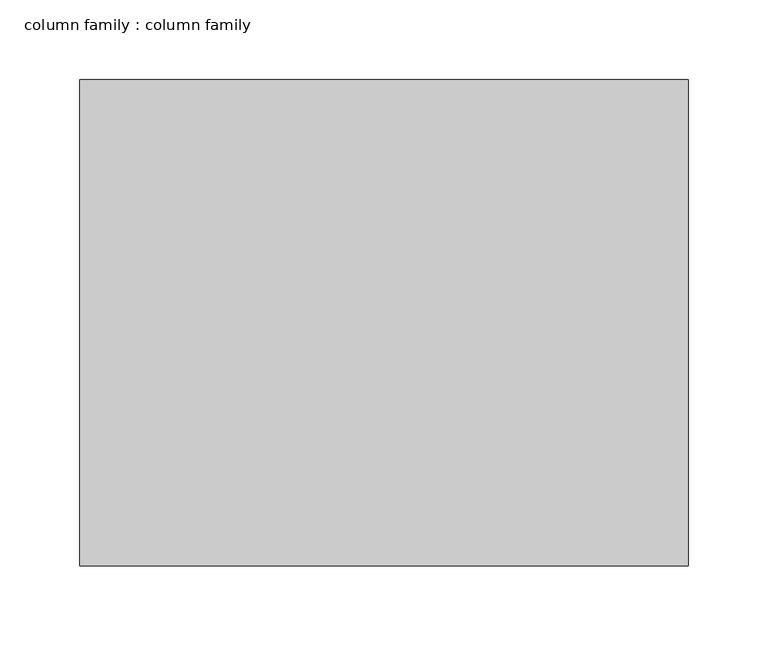
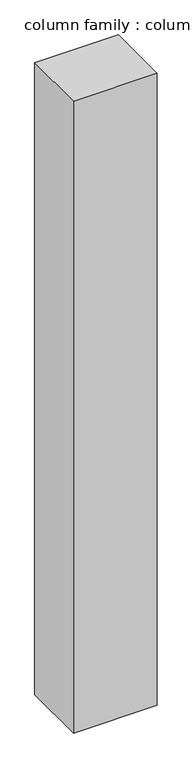
"""IFC4 building model written with IfcOpenShell, lengths in millimetres: column geometry, column family : column family."""

from ifc_helpers import new_model, si_unit, frame, origin, place, context, project, spatial, polyline, outline, extrude, source, transform, mapped, element, save


def column_family_column_family_eebd7f06(model_context):
    return source(origin(), model_context, "Body", "SweptSolid", [
        extrude(outline(polyline([(246.1278467, 152.4), (246.1278467, -152.4), (-134.8721533, -152.4), (-134.8721533, 152.4), (246.1278467, 152.4)])), frame((0.0, 0.0, 5.0), z_axis=(0.0, 0.0, 1.0), x_axis=(1.0, 0.0, 0.0)), (0.0, 0.0, 1.0), 3038.0),
    ])


if __name__ == "__main__":
    model = new_model("IFC4")
    model_context = context("Model", 3, world=origin())
    ifc_project = project(units=[si_unit("LENGTHUNIT", "METRE", prefix="MILLI")], contexts=[model_context])
    site = spatial("IfcSite", under=ifc_project)
    building = spatial("IfcBuilding", under=site)
    placement = place(None, origin())
    column_family_column_family_shape = column_family_column_family_eebd7f06(model_context)
    element("IfcColumn", 1, ObjectType="column family : column family", at=placement, inside=building, context=model_context, shape_type="MappedRepresentation", body=[
        mapped(column_family_column_family_shape, transform((0.0, 0.0, 0.0), x_axis=(1.0, 0.0, 0.0), y_axis=(0.0, 1.0, 0.0), z_axis=(0.0, 0.0, 1.0))),
    ])
    save(model, "model.ifc")

# Revit data of these elements
# Type "column family : column family"
#   w2 [instance default] = 0' - 9.88189"
#   w1 [instance default] = 0' - 9.01575"
#   Depth = 1' - 11.62205"
#   Width = 1' - 11.62205"
# Element 1 (IfcColumn, "column family : column family")
#   w2 = 1' - 0"
#   w1 = 1' - 3"
